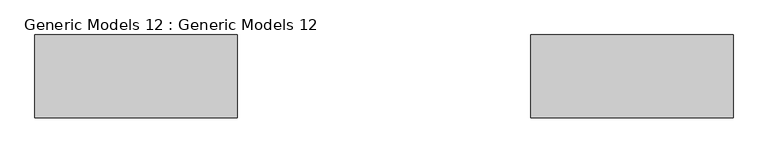
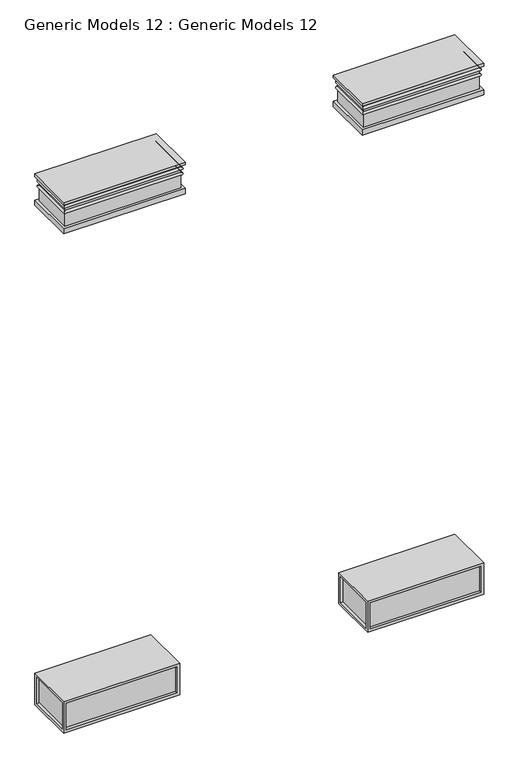
"""IFC4 building model written with IfcOpenShell, lengths in millimetres: proxy geometry, Generic Models 12 : Generic Models 12."""

from ifc_helpers import new_model, si_unit, frame, origin, place, context, project, spatial, ellipse_curve, faceted_brep, source, transform, mapped, element, save
from ifc_brep_helpers import plane_surface, cylinder_surface, advanced_brep


def generic_models_12_generic_models_12_08b21b51(model_context):
    return source(origin(), model_context, "Body", "SolidModel", [
        advanced_brep(
        [(-99.8825076, -7323.0292912, 4851.4), (1017.7174924, -7323.0292912, 4851.4), (1017.7174924, -7780.2292912, 4851.4), (-99.8825076, -7780.2292912, 4851.4), (-99.8825076, -7323.0292912, 5156.2), (-99.8825076, -7780.2292912, 5156.2), (1017.7174924, -7780.2292912, 5156.2), (1017.7174924, -7323.0292912, 5156.2), (-99.8825076, -7780.2292912, 4902.2), (-99.8825076, -7323.0292912, 4902.2), (-99.8825076, -7323.0292912, 5130.3285072), (-99.8825076, -7780.2292912, 5130.3285072), (1017.7174924, -7780.2292912, 4902.2), (1017.7174924, -7780.2292912, 5130.3285072), (1017.7174924, -7323.0292912, 4902.2), (1017.7174924, -7323.0292912, 5130.3285072), (992.3174924, -7754.8292912, 5105.4), (992.3174924, -7348.4292912, 5105.4), (992.3174924, -7348.4292912, 5130.3285072), (992.3174924, -7754.8292912, 5130.3285072), (992.3174924, -7754.8292912, 5080.0), (992.3174924, -7348.4292912, 5080.0), (992.3174924, -7754.8292912, 5054.6), (992.3174924, -7348.4292912, 5054.6), (992.3174924, -7754.8292912, 5029.2), (992.3174924, -7348.4292912, 5029.2), (992.3174924, -7754.8292912, 4902.2), (992.3174924, -7348.4292912, 4902.2), (-74.4825076, -7348.4292912, 5105.4), (-74.4825076, -7348.4292912, 5130.3285072), (-74.4825076, -7348.4292912, 5080.0), (-74.4825076, -7348.4292912, 5054.6), (-74.4825076, -7348.4292912, 5029.2), (-74.4825076, -7348.4292912, 4902.2), (-74.4825076, -7754.8292912, 5105.4), (-74.4825076, -7754.8292912, 5130.3285072), (-74.4825076, -7754.8292912, 5080.0), (-74.4825076, -7754.8292912, 5054.6), (-74.4825076, -7754.8292912, 5029.2), (-74.4825076, -7754.8292912, 4902.2)],
        [
            (0, 1),
            (1, 2),
            (2, 3),
            (3, 0),
            (4, 5),
            (5, 6),
            (6, 7),
            (7, 4),
            (3, 8),
            (8, 9),
            (9, 0),
            (4, 10),
            (10, 11),
            (11, 5),
            (2, 12),
            (12, 8),
            (11, 13),
            (13, 6),
            (1, 14),
            (14, 12),
            (13, 15),
            (15, 7),
            (9, 14),
            (15, 10),
            (16, 17),
            (17, 18),
            (18, 19),
            (19, 16),
            (16, 20, ellipse_curve(frame((992.3174924, -7754.8292912, 5092.7), z_axis=(0.707106781186549, 0.7071067811865461, 0.0), x_axis=(-0.7071067811865461, 0.7071067811865488, 0.0)), 17.9605122, 12.7)),
            (20, 21),
            (21, 17, ellipse_curve(frame((992.3174924, -7348.4292912, 5092.7), z_axis=(0.707106781186546, -0.707106781186549, 0.0), x_axis=(0.707106781186549, 0.707106781186546, 0.0)), 17.9605122, 12.7)),
            (20, 22),
            (22, 23),
            (23, 21),
            (22, 24, ellipse_curve(frame((992.3174924, -7754.8292912, 5041.9), z_axis=(0.707106781186549, 0.7071067811865461, 0.0), x_axis=(-0.7071067811865461, 0.7071067811865488, 0.0)), 17.9605122, 12.7)),
            (24, 25),
            (25, 23, ellipse_curve(frame((992.3174924, -7348.4292912, 5041.9), z_axis=(0.707106781186546, -0.707106781186549, 0.0), x_axis=(0.707106781186549, 0.707106781186546, 0.0)), 17.9605122, 12.7)),
            (24, 26),
            (26, 27),
            (27, 25),
            (17, 28),
            (28, 29),
            (29, 18),
            (21, 30),
            (30, 28, ellipse_curve(frame((-74.4825076, -7348.4292912, 5092.7), z_axis=(0.7071067811865492, 0.7071067811865457, 0.0), x_axis=(-0.7071067811865459, 0.7071067811865491, 0.0)), 17.9605122, 12.7)),
            (23, 31),
            (31, 30),
            (25, 32),
            (32, 31, ellipse_curve(frame((-74.4825076, -7348.4292912, 5041.9), z_axis=(0.7071067811865492, 0.7071067811865457, 0.0), x_axis=(-0.7071067811865459, 0.7071067811865491, 0.0)), 17.9605122, 12.7)),
            (27, 33),
            (33, 32),
            (28, 34),
            (34, 35),
            (35, 29),
            (30, 36),
            (36, 34, ellipse_curve(frame((-74.4825076, -7754.8292912, 5092.7), z_axis=(-0.7071067811865458, 0.7071067811865492, 0.0), x_axis=(-0.7071067811865492, -0.7071067811865458, 0.0)), 17.9605122, 12.7)),
            (31, 37),
            (37, 36),
            (32, 38),
            (38, 37, ellipse_curve(frame((-74.4825076, -7754.8292912, 5041.9), z_axis=(-0.7071067811865458, 0.7071067811865492, 0.0), x_axis=(-0.7071067811865492, -0.7071067811865458, 0.0)), 17.9605122, 12.7)),
            (33, 39),
            (39, 38),
            (19, 35),
            (34, 16),
            (36, 20),
            (37, 22),
            (38, 24),
            (39, 26),
        ],
        [
            plane_surface(frame((-99.8825076, -7780.2292912, 4851.4), z_axis=(0.0, 0.0, -1.0), x_axis=(0.0, 1.0, 0.0))),
            plane_surface(frame((-99.8825076, -7780.2292912, 5156.2), z_axis=(0.0, 0.0, 1.0), x_axis=(0.0, -1.0, 0.0))),
            plane_surface(frame((-99.8825076, -7323.0292912, 5156.2), z_axis=(-1.0, 0.0, 0.0), x_axis=(0.0, 0.0, -1.0))),
            plane_surface(frame((-99.8825076, -7780.2292912, 5156.2), z_axis=(0.0, -1.0, 0.0), x_axis=(0.0, 0.0, -1.0))),
            plane_surface(frame((1017.7174924, -7780.2292912, 5156.2), z_axis=(1.0, 0.0, 0.0), x_axis=(0.0, 0.0, -1.0))),
            plane_surface(frame((1017.7174924, -7323.0292912, 5156.2), z_axis=(0.0, 1.0, 0.0), x_axis=(0.0, 0.0, -1.0))),
            plane_surface(frame((992.3174924, -7754.8292912, 5130.3285072), z_axis=(1.0, 0.0, 0.0), x_axis=(0.0, 1.0, 0.0))),
            cylinder_surface(frame((992.3174924, -7780.2292912, 5092.7), z_axis=(0.0, 1.0, 0.0), x_axis=(-1.0, 0.0, 0.0)), 12.7),
            plane_surface(frame((992.3174924, -7754.8292912, 5080.0), z_axis=(1.0, 0.0, 0.0), x_axis=(0.0, 1.0, 0.0))),
            cylinder_surface(frame((992.3174924, -7780.2292912, 5041.9), z_axis=(0.0, 1.0, 0.0), x_axis=(-1.0, 0.0, 0.0)), 12.7),
            plane_surface(frame((992.3174924, -7754.8292912, 5029.2), z_axis=(1.0, 0.0, 0.0), x_axis=(0.0, 1.0, 0.0))),
            plane_surface(frame((992.3174924, -7348.4292912, 5130.3285072), z_axis=(0.0, 1.0, 0.0), x_axis=(-1.0, 0.0, 0.0))),
            cylinder_surface(frame((1017.7174924, -7348.4292912, 5092.7), z_axis=(-1.0, 0.0, 0.0), x_axis=(0.0, -1.0, 0.0)), 12.7),
            plane_surface(frame((992.3174924, -7348.4292912, 5080.0), z_axis=(0.0, 1.0, 0.0), x_axis=(-1.0, 0.0, 0.0))),
            cylinder_surface(frame((1017.7174924, -7348.4292912, 5041.9), z_axis=(-1.0, 0.0, 0.0), x_axis=(0.0, -1.0, 0.0)), 12.7),
            plane_surface(frame((992.3174924, -7348.4292912, 5029.2), z_axis=(0.0, 1.0, 0.0), x_axis=(-1.0, 0.0, 0.0))),
            plane_surface(frame((-74.4825076, -7348.4292912, 5130.3285072), z_axis=(-1.0, 0.0, 0.0), x_axis=(0.0, -1.0, 0.0))),
            cylinder_surface(frame((-74.4825076, -7323.0292912, 5092.7), z_axis=(0.0, -1.0, 0.0), x_axis=(1.0, 0.0, 0.0)), 12.7),
            plane_surface(frame((-74.4825076, -7348.4292912, 5080.0), z_axis=(-1.0, 0.0, 0.0), x_axis=(0.0, -1.0, 0.0))),
            cylinder_surface(frame((-74.4825076, -7323.0292912, 5041.9), z_axis=(0.0, -1.0, 0.0), x_axis=(1.0, 0.0, 0.0)), 12.7),
            plane_surface(frame((-74.4825076, -7348.4292912, 5029.2), z_axis=(-1.0, 0.0, 0.0), x_axis=(0.0, -1.0, 0.0))),
            plane_surface(frame((-74.4825076, -7754.8292912, 5130.3285072), z_axis=(0.0, -1.0, 0.0), x_axis=(1.0, 0.0, 0.0))),
            cylinder_surface(frame((-99.8825076, -7754.8292912, 5092.7), z_axis=(1.0, 0.0, 0.0), x_axis=(0.0, 1.0, 0.0)), 12.7),
            plane_surface(frame((-74.4825076, -7754.8292912, 5080.0), z_axis=(0.0, -1.0, 0.0), x_axis=(1.0, 0.0, 0.0))),
            cylinder_surface(frame((-99.8825076, -7754.8292912, 5041.9), z_axis=(1.0, 0.0, 0.0), x_axis=(0.0, 1.0, 0.0)), 12.7),
            plane_surface(frame((-74.4825076, -7754.8292912, 5029.2), z_axis=(0.0, -1.0, 0.0), x_axis=(1.0, 0.0, 0.0))),
            plane_surface(frame((-74.4825076, -7754.8292912, 4902.2), z_axis=(0.0, 0.0, 1.0), x_axis=(1.0, 0.0, 0.0))),
            plane_surface(frame((-99.8825076, -7780.2292912, 5130.3285072), z_axis=(0.0, 0.0, -1.0), x_axis=(1.0, 0.0, 0.0))),
        ],
        [
            (0, [[1, 2, 3, 4]]),
            (1, [[5, 6, 7, 8]]),
            (2, [[-4, 9, 10, 11]]),
            (2, [[-5, 12, 13, 14]]),
            (3, [[-3, 15, 16, -9]]),
            (3, [[-6, -14, 17, 18]]),
            (4, [[-2, 19, 20, -15]]),
            (4, [[-7, -18, 21, 22]]),
            (5, [[-1, -11, 23, -19]]),
            (5, [[-8, -22, 24, -12]]),
            (6, [[25, 26, 27, 28]]),
            (7, [[-25, 29, 30, 31]]),
            (8, [[-30, 32, 33, 34]]),
            (9, [[-33, 35, 36, 37]]),
            (10, [[-36, 38, 39, 40]]),
            (11, [[-26, 41, 42, 43]]),
            (12, [[-31, 44, 45, -41]]),
            (13, [[-34, 46, 47, -44]]),
            (14, [[-37, 48, 49, -46]]),
            (15, [[-40, 50, 51, -48]]),
            (16, [[-42, 52, 53, 54]]),
            (17, [[-45, 55, 56, -52]]),
            (18, [[-47, 57, 58, -55]]),
            (19, [[-49, 59, 60, -57]]),
            (20, [[-51, 61, 62, -59]]),
            (21, [[-28, 63, -53, 64]]),
            (22, [[-29, -64, -56, 65]]),
            (23, [[-32, -65, -58, 66]]),
            (24, [[-35, -66, -60, 67]]),
            (25, [[-38, -67, -62, 68]]),
            (26, [[-10, -16, -20, -23], [-39, -68, -61, -50]]),
            (27, [[-13, -24, -21, -17], [-27, -43, -54, -63]]),
        ],
    ),
        advanced_brep(
        [(-2843.0825076, -7323.0292912, 4851.4), (-1725.4825076, -7323.0292912, 4851.4), (-1725.4825076, -7780.2292912, 4851.4), (-2843.0825076, -7780.2292912, 4851.4), (-2843.0825076, -7323.0292912, 5156.2), (-2843.0825076, -7780.2292912, 5156.2), (-1725.4825076, -7780.2292912, 5156.2), (-1725.4825076, -7323.0292912, 5156.2), (-2843.0825076, -7780.2292912, 4902.2), (-2843.0825076, -7323.0292912, 4902.2), (-2843.0825076, -7323.0292912, 5130.3285072), (-2843.0825076, -7780.2292912, 5130.3285072), (-1725.4825076, -7780.2292912, 4902.2), (-1725.4825076, -7780.2292912, 5130.3285072), (-1725.4825076, -7323.0292912, 4902.2), (-1725.4825076, -7323.0292912, 5130.3285072), (-1750.8825076, -7754.8292912, 5105.4), (-1750.8825076, -7348.4292912, 5105.4), (-1750.8825076, -7348.4292912, 5130.3285072), (-1750.8825076, -7754.8292912, 5130.3285072), (-1750.8825076, -7754.8292912, 5080.0), (-1750.8825076, -7348.4292912, 5080.0), (-1750.8825076, -7754.8292912, 5054.6), (-1750.8825076, -7348.4292912, 5054.6), (-1750.8825076, -7754.8292912, 5029.2), (-1750.8825076, -7348.4292912, 5029.2), (-1750.8825076, -7754.8292912, 4902.2), (-1750.8825076, -7348.4292912, 4902.2), (-2817.6825076, -7348.4292912, 5105.4), (-2817.6825076, -7348.4292912, 5130.3285072), (-2817.6825076, -7348.4292912, 5080.0), (-2817.6825076, -7348.4292912, 5054.6), (-2817.6825076, -7348.4292912, 5029.2), (-2817.6825076, -7348.4292912, 4902.2), (-2817.6825076, -7754.8292912, 5105.4), (-2817.6825076, -7754.8292912, 5130.3285072), (-2817.6825076, -7754.8292912, 5080.0), (-2817.6825076, -7754.8292912, 5054.6), (-2817.6825076, -7754.8292912, 5029.2), (-2817.6825076, -7754.8292912, 4902.2)],
        [
            (0, 1),
            (1, 2),
            (2, 3),
            (3, 0),
            (4, 5),
            (5, 6),
            (6, 7),
            (7, 4),
            (3, 8),
            (8, 9),
            (9, 0),
            (4, 10),
            (10, 11),
            (11, 5),
            (2, 12),
            (12, 8),
            (11, 13),
            (13, 6),
            (1, 14),
            (14, 12),
            (13, 15),
            (15, 7),
            (9, 14),
            (15, 10),
            (16, 17),
            (17, 18),
            (18, 19),
            (19, 16),
            (16, 20, ellipse_curve(frame((-1750.8825076, -7754.8292912, 5092.7), z_axis=(0.707106781186549, 0.7071067811865461, 0.0), x_axis=(-0.7071067811865461, 0.7071067811865488, 0.0)), 17.9605122, 12.7)),
            (20, 21),
            (21, 17, ellipse_curve(frame((-1750.8825076, -7348.4292912, 5092.7), z_axis=(0.707106781186546, -0.707106781186549, 0.0), x_axis=(0.707106781186549, 0.707106781186546, 0.0)), 17.9605122, 12.7)),
            (20, 22),
            (22, 23),
            (23, 21),
            (22, 24, ellipse_curve(frame((-1750.8825076, -7754.8292912, 5041.9), z_axis=(0.707106781186549, 0.7071067811865461, 0.0), x_axis=(-0.7071067811865461, 0.7071067811865488, 0.0)), 17.9605122, 12.7)),
            (24, 25),
            (25, 23, ellipse_curve(frame((-1750.8825076, -7348.4292912, 5041.9), z_axis=(0.707106781186546, -0.707106781186549, 0.0), x_axis=(0.707106781186549, 0.707106781186546, 0.0)), 17.9605122, 12.7)),
            (24, 26),
            (26, 27),
            (27, 25),
            (17, 28),
            (28, 29),
            (29, 18),
            (21, 30),
            (30, 28, ellipse_curve(frame((-2817.6825076, -7348.4292912, 5092.7), z_axis=(0.7071067811865492, 0.7071067811865457, 0.0), x_axis=(-0.7071067811865459, 0.7071067811865491, 0.0)), 17.9605122, 12.7)),
            (23, 31),
            (31, 30),
            (25, 32),
            (32, 31, ellipse_curve(frame((-2817.6825076, -7348.4292912, 5041.9), z_axis=(0.7071067811865492, 0.7071067811865457, 0.0), x_axis=(-0.7071067811865459, 0.7071067811865491, 0.0)), 17.9605122, 12.7)),
            (27, 33),
            (33, 32),
            (28, 34),
            (34, 35),
            (35, 29),
            (30, 36),
            (36, 34, ellipse_curve(frame((-2817.6825076, -7754.8292912, 5092.7), z_axis=(-0.7071067811865458, 0.7071067811865492, 0.0), x_axis=(-0.7071067811865492, -0.7071067811865458, 0.0)), 17.9605122, 12.7)),
            (31, 37),
            (37, 36),
            (32, 38),
            (38, 37, ellipse_curve(frame((-2817.6825076, -7754.8292912, 5041.9), z_axis=(-0.7071067811865458, 0.7071067811865492, 0.0), x_axis=(-0.7071067811865492, -0.7071067811865458, 0.0)), 17.9605122, 12.7)),
            (33, 39),
            (39, 38),
            (19, 35),
            (34, 16),
            (36, 20),
            (37, 22),
            (38, 24),
            (39, 26),
        ],
        [
            plane_surface(frame((-2843.0825076, -7780.2292912, 4851.4), z_axis=(0.0, 0.0, -1.0), x_axis=(0.0, 1.0, 0.0))),
            plane_surface(frame((-2843.0825076, -7780.2292912, 5156.2), z_axis=(0.0, 0.0, 1.0), x_axis=(0.0, -1.0, 0.0))),
            plane_surface(frame((-2843.0825076, -7323.0292912, 5156.2), z_axis=(-1.0, 0.0, 0.0), x_axis=(0.0, 0.0, -1.0))),
            plane_surface(frame((-2843.0825076, -7780.2292912, 5156.2), z_axis=(0.0, -1.0, 0.0), x_axis=(0.0, 0.0, -1.0))),
            plane_surface(frame((-1725.4825076, -7780.2292912, 5156.2), z_axis=(1.0, 0.0, 0.0), x_axis=(0.0, 0.0, -1.0))),
            plane_surface(frame((-1725.4825076, -7323.0292912, 5156.2), z_axis=(0.0, 1.0, 0.0), x_axis=(0.0, 0.0, -1.0))),
            plane_surface(frame((-1750.8825076, -7754.8292912, 5130.3285072), z_axis=(1.0, 0.0, 0.0), x_axis=(0.0, 1.0, 0.0))),
            cylinder_surface(frame((-1750.8825076, -7780.2292912, 5092.7), z_axis=(0.0, 1.0, 0.0), x_axis=(-1.0, 0.0, 0.0)), 12.7),
            plane_surface(frame((-1750.8825076, -7754.8292912, 5080.0), z_axis=(1.0, 0.0, 0.0), x_axis=(0.0, 1.0, 0.0))),
            cylinder_surface(frame((-1750.8825076, -7780.2292912, 5041.9), z_axis=(0.0, 1.0, 0.0), x_axis=(-1.0, 0.0, 0.0)), 12.7),
            plane_surface(frame((-1750.8825076, -7754.8292912, 5029.2), z_axis=(1.0, 0.0, 0.0), x_axis=(0.0, 1.0, 0.0))),
            plane_surface(frame((-1750.8825076, -7348.4292912, 5130.3285072), z_axis=(0.0, 1.0, 0.0), x_axis=(-1.0, 0.0, 0.0))),
            cylinder_surface(frame((-1725.4825076, -7348.4292912, 5092.7), z_axis=(-1.0, 0.0, 0.0), x_axis=(0.0, -1.0, 0.0)), 12.7),
            plane_surface(frame((-1750.8825076, -7348.4292912, 5080.0), z_axis=(0.0, 1.0, 0.0), x_axis=(-1.0, 0.0, 0.0))),
            cylinder_surface(frame((-1725.4825076, -7348.4292912, 5041.9), z_axis=(-1.0, 0.0, 0.0), x_axis=(0.0, -1.0, 0.0)), 12.7),
            plane_surface(frame((-1750.8825076, -7348.4292912, 5029.2), z_axis=(0.0, 1.0, 0.0), x_axis=(-1.0, 0.0, 0.0))),
            plane_surface(frame((-2817.6825076, -7348.4292912, 5130.3285072), z_axis=(-1.0, 0.0, 0.0), x_axis=(0.0, -1.0, 0.0))),
            cylinder_surface(frame((-2817.6825076, -7323.0292912, 5092.7), z_axis=(0.0, -1.0, 0.0), x_axis=(1.0, 0.0, 0.0)), 12.7),
            plane_surface(frame((-2817.6825076, -7348.4292912, 5080.0), z_axis=(-1.0, 0.0, 0.0), x_axis=(0.0, -1.0, 0.0))),
            cylinder_surface(frame((-2817.6825076, -7323.0292912, 5041.9), z_axis=(0.0, -1.0, 0.0), x_axis=(1.0, 0.0, 0.0)), 12.7),
            plane_surface(frame((-2817.6825076, -7348.4292912, 5029.2), z_axis=(-1.0, 0.0, 0.0), x_axis=(0.0, -1.0, 0.0))),
            plane_surface(frame((-2817.6825076, -7754.8292912, 5130.3285072), z_axis=(0.0, -1.0, 0.0), x_axis=(1.0, 0.0, 0.0))),
            cylinder_surface(frame((-2843.0825076, -7754.8292912, 5092.7), z_axis=(1.0, 0.0, 0.0), x_axis=(0.0, 1.0, 0.0)), 12.7),
            plane_surface(frame((-2817.6825076, -7754.8292912, 5080.0), z_axis=(0.0, -1.0, 0.0), x_axis=(1.0, 0.0, 0.0))),
            cylinder_surface(frame((-2843.0825076, -7754.8292912, 5041.9), z_axis=(1.0, 0.0, 0.0), x_axis=(0.0, 1.0, 0.0)), 12.7),
            plane_surface(frame((-2817.6825076, -7754.8292912, 5029.2), z_axis=(0.0, -1.0, 0.0), x_axis=(1.0, 0.0, 0.0))),
            plane_surface(frame((-2817.6825076, -7754.8292912, 4902.2), z_axis=(0.0, 0.0, 1.0), x_axis=(1.0, 0.0, 0.0))),
            plane_surface(frame((-2843.0825076, -7780.2292912, 5130.3285072), z_axis=(0.0, 0.0, -1.0), x_axis=(1.0, 0.0, 0.0))),
        ],
        [
            (0, [[1, 2, 3, 4]]),
            (1, [[5, 6, 7, 8]]),
            (2, [[-4, 9, 10, 11]]),
            (2, [[-5, 12, 13, 14]]),
            (3, [[-3, 15, 16, -9]]),
            (3, [[-6, -14, 17, 18]]),
            (4, [[-2, 19, 20, -15]]),
            (4, [[-7, -18, 21, 22]]),
            (5, [[-1, -11, 23, -19]]),
            (5, [[-8, -22, 24, -12]]),
            (6, [[25, 26, 27, 28]]),
            (7, [[-25, 29, 30, 31]]),
            (8, [[-30, 32, 33, 34]]),
            (9, [[-33, 35, 36, 37]]),
            (10, [[-36, 38, 39, 40]]),
            (11, [[-26, 41, 42, 43]]),
            (12, [[-31, 44, 45, -41]]),
            (13, [[-34, 46, 47, -44]]),
            (14, [[-37, 48, 49, -46]]),
            (15, [[-40, 50, 51, -48]]),
            (16, [[-42, 52, 53, 54]]),
            (17, [[-45, 55, 56, -52]]),
            (18, [[-47, 57, 58, -55]]),
            (19, [[-49, 59, 60, -57]]),
            (20, [[-51, 61, 62, -59]]),
            (21, [[-28, 63, -53, 64]]),
            (22, [[-29, -64, -56, 65]]),
            (23, [[-32, -65, -58, 66]]),
            (24, [[-35, -66, -60, 67]]),
            (25, [[-38, -67, -62, 68]]),
            (26, [[-10, -16, -20, -23], [-39, -68, -61, -50]]),
            (27, [[-13, -24, -21, -17], [-27, -43, -54, -63]]),
        ],
    ),
        faceted_brep([(-1776.2825076, -7780.2292912, 304.8), (-1776.2825076, -7323.0292912, 304.8), (-2843.0825076, -7323.0292912, 304.8), (-2843.0825076, -7780.2292912, 304.8), (-1776.2825076, -7780.2292912, 0.0), (-2843.0825076, -7780.2292912, 0.0), (-2843.0825076, -7323.0292912, 0.0), (-1776.2825076, -7323.0292912, 0.0), (-1776.2825076, -7348.4292912, 279.4), (-1776.2825076, -7348.4292912, 25.4), (-1776.2825076, -7754.8292912, 25.4), (-1776.2825076, -7754.8292912, 279.4), (-2843.0825076, -7754.8292912, 279.4), (-2843.0825076, -7754.8292912, 25.4), (-2843.0825076, -7348.4292912, 25.4), (-2843.0825076, -7348.4292912, 279.4), (-2817.6825076, -7780.2292912, 279.4), (-1801.6825076, -7780.2292912, 279.4), (-1801.6825076, -7780.2292912, 25.4), (-2817.6825076, -7780.2292912, 25.4), (-2817.6825076, -7754.8292912, 279.4), (-2817.6825076, -7754.8292912, 25.4), (-1801.6825076, -7754.8292912, 25.4), (-1801.6825076, -7754.8292912, 279.4), (-2817.6825076, -7754.8292912, 279.4), (-2817.6825076, -7348.4292912, 279.4), (-2817.6825076, -7348.4292912, 25.4), (-2817.6825076, -7754.8292912, 25.4), (-1801.6825076, -7348.4292912, 279.4), (-1801.6825076, -7754.8292912, 279.4), (-1801.6825076, -7754.8292912, 25.4), (-1801.6825076, -7348.4292912, 25.4)], [[[0, 1, 2, 3]], [[4, 5, 6, 7]], [[1, 0, 4, 7], [8, 9, 10, 11]], [[2, 1, 7, 6]], [[3, 2, 6, 5], [12, 13, 14, 15]], [[0, 3, 5, 4], [16, 17, 18, 19]], [[20, 21, 22, 23]], [[20, 23, 17, 16]], [[23, 22, 18, 17]], [[22, 21, 19, 18]], [[21, 20, 16, 19]], [[24, 25, 26, 27]], [[24, 27, 13, 12]], [[27, 26, 14, 13]], [[26, 25, 15, 14]], [[25, 24, 12, 15]], [[28, 29, 30, 31]], [[28, 31, 9, 8]], [[31, 30, 10, 9]], [[30, 29, 11, 10]], [[29, 28, 8, 11]]]),
        faceted_brep([(-49.0825076, -7780.2292912, 304.8), (1017.7174924, -7780.2292912, 304.8), (1017.7174924, -7323.0292912, 304.8), (-49.0825076, -7323.0292912, 304.8), (-49.0825076, -7780.2292912, 0.0), (-49.0825076, -7323.0292912, 0.0), (1017.7174924, -7323.0292912, 0.0), (1017.7174924, -7780.2292912, 0.0), (-23.6825076, -7780.2292912, 279.4), (992.3174924, -7780.2292912, 279.4), (992.3174924, -7780.2292912, 25.4), (-23.6825076, -7780.2292912, 25.4), (1017.7174924, -7348.4292912, 279.4), (1017.7174924, -7348.4292912, 25.4), (1017.7174924, -7754.8292912, 25.4), (1017.7174924, -7754.8292912, 279.4), (-49.0825076, -7754.8292912, 279.4), (-49.0825076, -7754.8292912, 25.4), (-49.0825076, -7348.4292912, 25.4), (-49.0825076, -7348.4292912, 279.4), (-23.6825076, -7754.8292912, 279.4), (-23.6825076, -7754.8292912, 25.4), (992.3174924, -7754.8292912, 25.4), (992.3174924, -7754.8292912, 279.4), (-23.6825076, -7754.8292912, 279.4), (-23.6825076, -7348.4292912, 279.4), (-23.6825076, -7348.4292912, 25.4), (-23.6825076, -7754.8292912, 25.4), (992.3174924, -7348.4292912, 279.4), (992.3174924, -7754.8292912, 279.4), (992.3174924, -7754.8292912, 25.4), (992.3174924, -7348.4292912, 25.4)], [[[0, 1, 2, 3]], [[4, 5, 6, 7]], [[1, 0, 4, 7], [8, 9, 10, 11]], [[2, 1, 7, 6], [12, 13, 14, 15]], [[3, 2, 6, 5]], [[0, 3, 5, 4], [16, 17, 18, 19]], [[20, 21, 22, 23]], [[20, 23, 9, 8]], [[23, 22, 10, 9]], [[22, 21, 11, 10]], [[21, 20, 8, 11]], [[24, 25, 26, 27]], [[24, 27, 17, 16]], [[27, 26, 18, 17]], [[26, 25, 19, 18]], [[25, 24, 16, 19]], [[28, 29, 30, 31]], [[28, 31, 13, 12]], [[31, 30, 14, 13]], [[30, 29, 15, 14]], [[29, 28, 12, 15]]]),
    ])


if __name__ == "__main__":
    model = new_model("IFC4")
    model_context = context("Model", 3, world=origin())
    ifc_project = project(units=[si_unit("LENGTHUNIT", "METRE", prefix="MILLI")], contexts=[model_context])
    site = spatial("IfcSite", under=ifc_project)
    building = spatial("IfcBuilding", under=site)
    placement = place(None, origin())
    generic_models_12_generic_models_12_shape = generic_models_12_generic_models_12_08b21b51(model_context)
    element("IfcBuildingElementProxy", 1, Name="Generic Models 12 : Generic Models 12", ObjectType="Generic Models 12 : Generic Models 12", at=placement, inside=building, context=model_context, shape_type="MappedRepresentation", body=[
        mapped(generic_models_12_generic_models_12_shape, transform((0.0, 0.0, 0.0), x_axis=(1.0, 0.0, 0.0), y_axis=(0.0, 1.0, 0.0), z_axis=(0.0, 0.0, 1.0))),
    ])
    save(model, "model.ifc")
